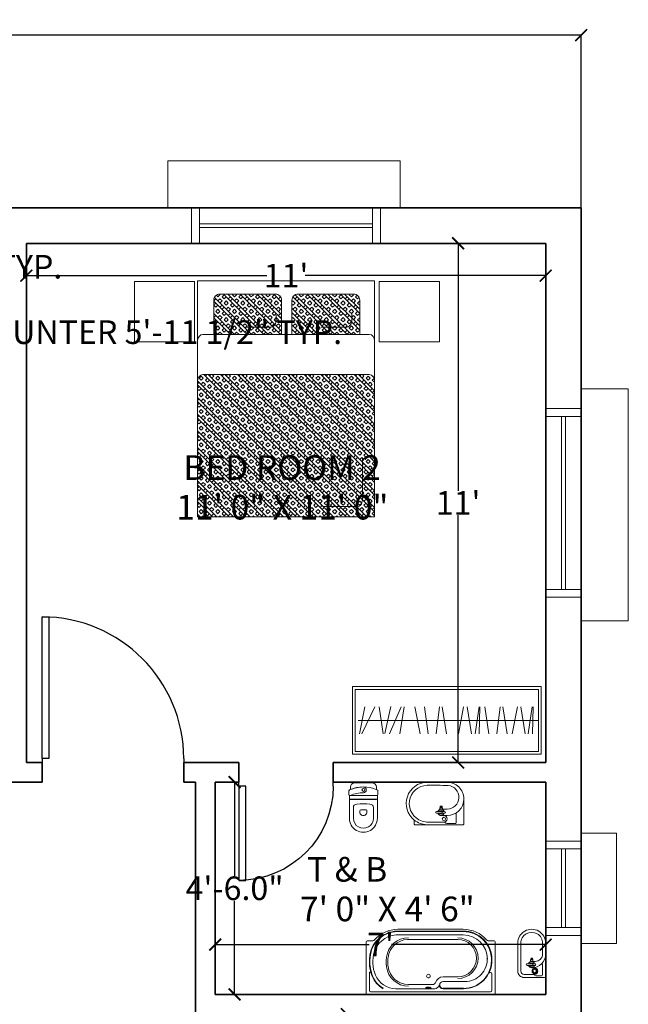
# Model space of a CAD drawing. Units: inches. Extents: x 844 to 2234, y 346 to 1084.
# Tile 93 of 93: x 2033 to 2188, y 828 to 1078. Entities that reach past the tile are written whole.
import ezdxf

# ---------------------------------------------------------------- set-up
doc = ezdxf.new("R2010")
doc.units = ezdxf.units.IN
doc.header["$MEASUREMENT"] = 0
for name, color, linetype, lineweight in [('A-ANNO-DIMS', 2, 'Continuous', 18), ('A-AREA-IDEN', 7, 'Continuous', 18), ('A-FLOR-FIXT', 8, 'Continuous', 18), ('A-WALL', 7, 'Continuous', 35), ('beds', 130, 'Continuous', 18), ('doors', 170, 'Continuous', 25), ('furniture', 8, 'Continuous', 18), ('windows', 1, 'Continuous', 18)]:
    doc.layers.add(name, color=color, linetype=linetype, lineweight=lineweight)
doc.styles.get("Standard").update_dxf_attribs({"font": 'arial.ttf'})
doc.dimstyles.get("Standard").update_dxf_attribs({"dimtxt": 6, "dimasz": 3, "dimexe": 0.18, "dimexo": 0.0625, "dimgap": 0.09, "dimtad": 0, "dimtih": 1, "dimtoh": 1, "dimdec": 1, "dimzin": 0, "dimdsep": 46, "dimlunit": 3, "dimtxsty": 'Standard', "dimblk": 'ARCHTICK', "dimcen": 0.09, "dimadec": 0, "dimazin": 0, "dimtfac": 1, "dimtdec": 1, "dimtofl": 0, "dimtmove": 0, "dimatfit": 3, "dimfxl": 1, "dimtolj": 1, "dimtzin": 0, "dimarcsym": 0})
pattern_1 = [(135, (-1377.70473, -125.71507), (-0.070710678, -0.070710678), []), (135, (-1377.68705, -125.69739), (-0.070710678, -0.070710678), []), (45, (-1377.70473, -125.71507), (-0.070710678, 0.070710678), [-0.025, 0.025]), (45, (-1377.72241, -125.69739), (-0.070710678, 0.070710678), [-0.025, 0.025]), (45, (-1377.74009, -125.67972), (-0.070710678, 0.070710678), [0.025, -0.025]), (45, (-1377.75776, -125.66204), (-0.070710678, 0.070710678), [0.025, -0.025]), (135, (-1377.66938, -125.67972), (-0.070710678, -0.070710678), [0.025, -0.025]), (135, (-1377.6517, -125.66204), (-0.070710678, -0.070710678), [0.025, -0.025])]

# ---------------------------------------------------------------- blocks, each defined once
blk = doc.blocks.new('*U2')
for p, q in [((0, 0), (0, -6)), ((36, 0), (36, -6))]:
    blk.add_line(p, q)
blk.add_lwpolyline([(0, 0), (0, 36), (1.75, 36), (1.75, 0)], close=True)
blk.add_arc((0, 0), 36, 0, 90)
blk = doc.blocks.new('*U4')
for p, q in [((0, 0), (0, -6)), ((24, 0), (24, -6))]:
    blk.add_line(p, q)
blk.add_lwpolyline([(0, 0), (0, 24), (1.75, 24), (1.75, 0)], close=True)
blk.add_arc((0, 0), 24, 0, 90)
blk = doc.blocks.new('MAT-P10')
h = blk.add_hatch()
h.set_pattern_fill('BOX', color=256, scale=0.1, angle=45, style=0)
h.set_pattern_definition(pattern_1)
h.paths.add_polyline_path([(-0.1565, 1.4605), (0.417, 1.4605), (0.417, 1.7513, 0.414214), (0.367, 1.8013), (-0.1065, 1.8013, 0.414214), (-0.1565, 1.7513)])
h.paths.add_polyline_path([(0.5052, 1.4604), (1.0792, 1.4604), (1.0792, 1.7513, 0.414214), (1.0292, 1.8013), (0.5552, 1.8013, 0.414214), (0.5052, 1.7513)])
h = blk.add_hatch()
h.set_pattern_fill('BOX', color=256, scale=0.1, angle=45, style=0)
h.set_pattern_definition(pattern_1)
edge = h.paths.add_edge_path()
edge.add_line((1.2049, -0.085), (1.2049, 1.0625))
edge.add_ellipse((1.1608, 1.0627), major_axis=(0, 0.0568), ratio=0.776379, start_angle=270, end_angle=360)
edge.add_line((1.1608, 1.1195), (-0.251, 1.1195))
edge.add_ellipse((-0.251, 1.0627), major_axis=(0, 0.0568), ratio=0.776379, start_angle=0, end_angle=88.13958)
edge.add_line((-0.2951, 1.0641), (-0.2951, -0.085))
edge.add_line((-0.2951, -0.085), (1.2049, -0.085))
for p, q in [((-0.251, 1.4605), (1.1608, 1.4604)), ((-0.251, 1.1195), (1.1608, 1.1195)), ((1.1017, 0.406), (1.1017, 0.0572)), ((1.0576, 0.0004), (0.7754, 0.0004))]:
    blk.add_line(p, q)
for points in [[(-0.8301, 1.9091), (-0.3191, 1.9091), (-0.3191, 1.3981), (-0.8301, 1.3981)], [(1.2049, -0.085), (-0.2951, -0.085), (-0.2951, 1.9151), (1.2049, 1.915)], [(1.2441, 1.9091), (1.755, 1.9091), (1.755, 1.3981), (1.2441, 1.3981)]]:
    blk.add_lwpolyline(points, close=True)
for points in [[(0.417, 1.4604), (0.417, 1.7513, 0.414214), (0.367, 1.8013), (-0.1065, 1.8013, 0.414214), (-0.1565, 1.7513), (-0.1565, 1.4604)], [(1.0792, 1.4603), (1.0792, 1.7513, 0.414214), (1.0292, 1.8013), (0.5552, 1.8013, 0.414214), (0.5052, 1.7513), (0.5052, 1.4604)], [(0.3702, 1.6242), (0.3702, 1.5715, -0.414214), (0.3202, 1.5215), (0.1113, 1.5215)], [(1.0117, 1.6438), (1.0117, 1.5715, -0.414214), (0.9617, 1.5215), (0.7528, 1.5215)]]:
    blk.add_lwpolyline(points, format="xyb")
at = {"extrusion": (0, 0, -1)}
for centre, start_param, end_param in [((-0.251, 1.4036), 4.712389, 6.283185), ((1.1608, 1.4036), 0, 1.570796), ((-0.251, 1.0627), 4.712389, 6.283185), ((1.1608, 1.0627), 0, 1.570796), ((1.0576, 0.0572), 1.570796, 3.141593), ((1.0576, 0.0572), 1.570796, 3.141593)]:
    blk.add_ellipse(centre, major_axis=(0, 0.0568), ratio=0.776379, start_param=start_param, end_param=end_param, dxfattribs=at)
blk = doc.blocks.new('A$C7A17768A')
for p, q in [((-2.8, 0), (0, 0)), ((-2.8, -1), (-2.8, 0)), ((0, -1), (0, 0)), ((-2.76, -0.04), (-0.04, -0.04)), ((-2.76, -0.96), (-2.76, -0.04)), ((-0.04, -0.96), (-0.04, -0.04)), ((-2.617, -0.3), (-2.694, -0.7)), ((-2.66, -0.7), (-2.466, -0.3)), ((-2.403, -0.3), (-2.342, -0.7)), ((-2.229, -0.296), (-2.317, -0.696)), ((-2.074, -0.3), (-2.25, -0.7)), ((-2.096, -0.7), (-2.033, -0.3)), ((-1.875, -0.3), (-1.796, -0.7)), ((-1.732, -0.3), (-1.675, -0.7)), ((-1.555, -0.7), (-1.507, -0.3)), ((-1.467, -0.3), (-1.403, -0.7)), ((-1.227, -0.7), (-1.151, -0.3)), ((-1.098, -0.3), (-1.034, -0.7)), ((-0.98, -0.7), (-0.921, -0.3)), ((-0.908, -0.3), (-0.919, -0.7)), ((-0.834, -0.3), (-0.777, -0.7)), ((-0.657, -0.7), (-0.61, -0.3)), ((-0.57, -0.3), (-0.505, -0.7)), ((-0.429, -0.7), (-0.353, -0.3)), ((-0.301, -0.3), (-0.237, -0.7)), ((-0.192, -0.7), (-0.133, -0.3)), ((-0.12, -0.3), (-0.131, -0.7)), ((-0.04, -0.5), (-2.716, -0.5)), ((-2.8, -1), (0, -1)), ((-2.76, -0.96), (-0.04, -0.96))]:
    blk.add_line(p, q)
blk = doc.blocks.new('2SABICO')
at = {"color": 0, "linetype": 'ByBlock'}
for p, q in [((0.478, 0.195), (0.089, 0.195)), ((0.478, 0.152), (0.089, 0.152)), ((0, 0.106), (0, 0)), ((0, 0), (0, -0.18)), ((0.043, -0.039), (0.043, 0.106)), ((0.135, 0), (0.135, -0.003)), ((0.168, 0.064), (0.168, -0.015)), ((0.192, 0.064), (0.192, -0.015)), ((0.221, 0.012), (0.222, 0.012)), ((0.223, 0.016), (0.223, -0.016)), ((0.224, 0.017), (0.245, 0.017)), ((0.246, 0.016), (0.246, -0.016)), ((0.25, 0.014), (0.246, 0.014)), ((0.26, 0.01), (0.268, 0.01)), ((0.268, -0.01), (0.268, 0.01)), ((0.268, 0.01), (0.269, 0.009)), ((0.269, -0.009), (0.269, 0.009)), ((0.023, -0.057), (0.023, -0.135)), ((0.135, 0), (0.135, -0.039)), ((0.168, -0.015), (0.192, -0.015)), ((0.168, -0.015), (0.168, -0.046)), ((0.192, -0.015), (0.192, -0.046)), ((0.221, -0.012), (0.222, -0.012)), ((0.224, -0.017), (0.245, -0.017)), ((0.225, -0.017), (0.225, -0.047)), ((0.25, -0.014), (0.246, -0.014)), ((0.26, -0.01), (0.268, -0.01)), ((0.268, -0.01), (0.269, -0.009)), ((0.015, -0.195), (0.478, -0.195)), ((0.038, -0.15), (0.179, -0.15)), ((0.33, -0.152), (0.478, -0.152))]:
    blk.add_line(p, q, dxfattribs=at)
for radius in [0.035, 0.023]:
    blk.add_circle((0.089, -0.039), radius, dxfattribs=at)
for centre, radius, start, end in [((0.089, 0.106), 0.089, 90, 180), ((0.089, 0.106), 0.046, 90, 180), ((0.478, 0), 0.195, 270, 90), ((0.478, 0), 0.152, 270, 90), ((0.18, 0), 0.045, 105.6643, 180), ((0.18, 0), 0.042, 106.8152, 252.6853), ((0.18, 0), 0.0235, 121.1327, 237.8651), ((0.18, 0.064), 0.0121, 0, 180), ((0.18, 0), 0.045, 17.0576, 74.3357), ((0.18, 0), 0.042, 287.3147, 73.1848), ((0.18, 0), 0.0235, 302.1349, 58.8673), ((0.221, 0.013), 0.001, 197.9471, 270), ((0.222, 0.013), 0.001, 270, 0), ((0.224, 0.016), 0.001, 90, 180), ((0.245, 0.016), 0.001, 0, 90), ((0.25, 0), 0.0143, 270, 90), ((0.041, -0.057), 0.018, 99.5941, 180), ((0.038, -0.135), 0.015, 180, 270), ((0.037, -0.033), 0.006, 279.5941, 0), ((0.089, -0.039), 0.046, 180, 360), ((0.326, -0.003), 0.191, 180, 270), ((0.18, -0.046), 0.0125, 180, 0), ((0.179, -0.14), 0.01, 270, 42.9682), ((0.221, -0.013), 0.001, 90, 162.0529), ((0.222, -0.013), 0.001, 0, 90), ((0.224, -0.016), 0.001, 180, 270), ((0.33, -0.047), 0.105, 180, 270), ((0.245, -0.016), 0.001, 270, 0), ((0.015, -0.18), 0.015, 180, 270)]:
    blk.add_arc(centre, radius, start, end, dxfattribs=at)
blk = doc.blocks.new('2SAINCO')
at = {"color": 0, "linetype": 'ByBlock'}
for p, q in [((0.06, 0.181), (0.085, 0.181)), ((0.114, 0.203), (0.165, 0.203)), ((0.496, 0.195), (0.178, 0.195)), ((0.18, -0.188), (0.18, 0.188)), ((0.231, 0.185), (0.231, -0.185)), ((0.234, 0.185), (0.234, -0.185)), ((0.496, 0.14), (0.347, 0.14)), ((0, -0.121), (0, 0.121)), ((0.394, 0.05), (0.407, 0.05)), ((0.394, -0.05), (0.407, -0.05)), ((0.06, -0.181), (0.085, -0.181)), ((0.114, -0.201), (0.165, -0.201)), ((0.114, -0.203), (0.165, -0.203)), ((0.496, -0.195), (0.178, -0.195)), ((0.496, -0.14), (0.347, -0.14))]:
    blk.add_line(p, q, dxfattribs=at)
blk.add_circle((0.1, 0), 0.02, dxfattribs=at)
for centre, radius, start, end in [((0.06, 0.121), 0.06, 90, 180), ((0.517, 0), 0.46, 155.909, 204.091), ((0.085, 0.196), 0.015, 270, 344.534), ((0.114, 0.188), 0.015, 90, 164.534), ((0.165, 0.188), 0.015, 0, 90), ((0.221, 0.185), 0.01, 0, 90), ((0.224, 0.185), 0.01, 0, 90), ((0.347, 0.09), 0.05, 90, 177.3546), ((0.496, 0), 0.195, 270, 90), ((0.496, 0), 0.14, 270, 90), ((0.1, 0), 0.0405, 360, 180), ((0.517, 0), 0.458, 180, 204.67), ((0.66, 0.008), 0.52, 180.891, 201.3823), ((2.295, 0), 2, 177.3546, 182.6454), ((0.677, 0), 0.3, 172.9459, 187.0541), ((0.394, 0.035), 0.015, 90, 172.9459), ((0.407, 0), 0.05, 270, 90), ((0.06, -0.121), 0.06, 180, 270), ((0.347, -0.09), 0.05, 182.6454, 270), ((0.394, -0.035), 0.015, 187.0541, 270), ((0.085, -0.196), 0.015, 15.466, 90), ((0.114, -0.188), 0.015, 195.466, 270), ((0.114, -0.188), 0.013, 195.466, 270), ((0.165, -0.188), 0.013, 270, 30), ((0.165, -0.188), 0.015, 270, 0), ((0.221, -0.185), 0.01, 270, 0), ((0.224, -0.185), 0.01, 270, 0)]:
    blk.add_arc(centre, radius, start, end, dxfattribs=at)
blk = doc.blocks.new('2SABACO')
at = {"color": 0}
for p, q in [((1.341, 0.831), (0.407, 0.831)), ((1.341, 0.91), (0.429, 0.91)), ((1.341, 0.885), (0.429, 0.885)), ((1.341, 0.879), (0.429, 0.879)), ((-0.015, 0.735), (-0.015, 0.015)), ((0, 0.75), (0.08, 0.75)), ((1.263, 0.769), (0.562, 0.769)), ((1.77, 0.75), (1.69, 0.75)), ((1.785, 0.015), (1.785, 0.735)), ((0.03, 0.302), (0.03, 0.053)), ((1.74, 0.053), (1.74, 0.286)), ((0.578, 0.139), (0.911, 0.139)), ((1.263, 0.245), (1.06, 0.245)), ((1.363, 0.181), (1.06, 0.181)), ((0, 0), (1.77, 0)), ((0.048, 0.035), (1.722, 0.035)), ((0.401, 0.08), (0.942, 0.08)), ((1.343, 0.086), (1.06, 0.086)), ((1.343, 0.079), (1.06, 0.079))]:
    blk.add_line(p, q, dxfattribs=at)
blk.add_circle((0.855, 0.256), 0.026, dxfattribs=at)
for centre, radius, start, end in [((0.428, 0.49), 0.395, 98.9726, 181.1954), ((0.428, 0.49), 0.389, 98.9726, 181.2301), ((0.425, 0.49), 0.342, 93.1008, 168.0202), ((0.429, 0.48), 0.43, 90, 139.2943), ((0.429, 0.48), 0.405, 90, 98.9726), ((0.429, 0.48), 0.399, 90, 98.9726), ((1.341, 0.48), 0.43, 40.7057, 90), ((1.341, 0.485), 0.401, 359.4627, 90), ((1.341, 0.485), 0.394, 3.5237, 90), ((1.341, 0.495), 0.336, 0, 90), ((0, 0.735), 0.015, 90, 180), ((0.08, 0.78), 0.03, 270, 319.2943), ((0.578, 0.481), 0.311, 90, 172.609), ((0.578, 0.481), 0.288, 93.3767, 172.609), ((1.263, 0.507), 0.285, 270, 90), ((1.263, 0.507), 0.262, 270, 90), ((1.69, 0.78), 0.03, 220.7057, 270), ((1.77, 0.735), 0.015, 0, 90), ((0.559, 0.454), 0.48, 163.1286, 202.3619), ((0.559, 0.454), 0.528, 177.0415, 202.3619), ((0.559, 0.454), 0.521, 177.0156, 202.3619), ((0.79, 0.454), 0.525, 172.609, 180), ((0.79, 0.454), 0.525, 180, 187.391), ((0.79, 0.454), 0.502, 172.609, 180), ((0.79, 0.454), 0.502, 180, 187.391), ((1.343, 0.477), 0.392, 270, 4.5675), ((1.343, 0.477), 0.398, 270, 0.539), ((1.363, 0.495), 0.314, 270, 2.2815), ((0.042, 0.302), 0.0116, 16.3184, 180.0001), ((0.578, 0.427), 0.311, 187.391, 270), ((0.578, 0.427), 0.288, 187.391, 270), ((1.718, 0.286), 0.0222, 0, 152.9966), ((0.401, 0.389), 0.357, 202.3619, 239.8287), ((0.401, 0.389), 0.351, 202.3619, 239.2093), ((0.401, 0.389), 0.309, 202.3619, 270), ((0.911, 0.183), 0.045, 270, 341.2369), ((1.06, 0.133), 0.112, 90, 161.2369), ((1.06, 0.133), 0.0475, 90, 270), ((0, 0.015), 0.015, 180, 270), ((0.048, 0.053), 0.018, 180, 270), ((0.559, 0.454), 0.48, 250.7818, 251.0555), ((0.821, 0.092), 0.00282, 119.7759, 180), ((0.821, 0.092), 0.00282, 180, 240.2241), ((0.837, 0.064), 0.0347, 103.3326, 119.7759), ((0.835, 0.025), 0.071, 96.5949, 102.1924), ((0.837, 0.12), 0.0347, 240.2241, 256.6674), ((0.847, -0.08), 0.177, 92.7417, 96.5949), ((0.848, 0.02), 0.0808, 95.6065, 103.3326), ((0.848, 0.164), 0.0808, 256.6674, 264.3935), ((0.855, -0.252), 0.349, 90, 92.7417), ((0.855, -0.053), 0.153, 90, 95.6065), ((0.855, 0.237), 0.153, 264.3935, 270), ((0.855, -0.053), 0.153, 84.3935, 90), ((0.855, -0.252), 0.349, 87.2583, 90), ((0.855, 0.237), 0.153, 270, 275.6065), ((0.862, 0.02), 0.0808, 76.6674, 84.3935), ((0.862, 0.164), 0.0808, 275.6065, 283.3326), ((0.863, -0.08), 0.177, 83.4051, 87.2583), ((0.873, 0.064), 0.0347, 60.2241, 76.6674), ((0.873, 0.12), 0.0347, 283.3326, 299.7759), ((0.875, 0.025), 0.071, 77.8076, 83.4051), ((0.889, 0.092), 0.00282, 360, 60.2241), ((0.889, 0.092), 0.00282, 299.7759, 360), ((0.942, 0.145), 0.065, 270, 349.4977), ((1.06, 0.133), 0.054, 180, 270), ((1.722, 0.053), 0.018, 270, 0), ((1.77, 0.015), 0.015, 270, 0)]:
    blk.add_arc(centre, radius, start, end, dxfattribs=at)
blk = doc.blocks.new('2SALACO2')
at = {"color": 0}
for p, q in [((0, 0), (-0.392, 0)), ((0.28, 0), (0, 0)), ((-0.402, -0.01), (-0.402, -0.36)), ((-0.293, -0.026), (-0.293, -0.15)), ((-0.283, -0.016), (-0.166, -0.016)), ((-0.169, -0.128), (-0.085, -0.128)), ((-0.112, -0.035), (-0.133, -0.035)), ((-0.124, -0.035), (0.09, -0.035)), ((0.29, -0.01), (0.29, -0.064)), ((-0.102, -0.219), (-0.169, -0.219)), ((-0.1, -0.161), (-0.131, -0.161)), ((-0.1, -0.186), (-0.131, -0.186)), ((-0.102, -0.217), (-0.102, -0.234)), ((-0.07, -0.216), (-0.101, -0.216)), ((-0.07, -0.235), (-0.101, -0.235)), ((-0.1, -0.161), (-0.1, -0.186)), ((-0.021, -0.161), (-0.1, -0.161)), ((-0.021, -0.186), (-0.1, -0.186)), ((-0.098, -0.214), (-0.098, -0.216)), ((-0.097, -0.239), (-0.098, -0.241)), ((-0.098, -0.241), (-0.098, -0.248)), ((-0.098, -0.241), (-0.073, -0.241)), ((-0.073, -0.248), (-0.098, -0.248)), ((-0.097, -0.235), (-0.097, -0.239)), ((-0.074, -0.239), (-0.097, -0.239)), ((-0.097, -0.248), (-0.097, -0.256)), ((-0.073, -0.256), (-0.097, -0.256)), ((-0.097, -0.256), (-0.094, -0.257)), ((-0.077, -0.257), (-0.094, -0.257)), ((-0.073, -0.256), (-0.077, -0.257)), ((-0.074, -0.235), (-0.074, -0.239)), ((-0.074, -0.239), (-0.073, -0.241)), ((-0.073, -0.214), (-0.073, -0.216)), ((-0.073, -0.241), (-0.073, -0.248)), ((-0.073, -0.248), (-0.073, -0.256)), ((-0.069, -0.217), (-0.069, -0.234))]:
    blk.add_line(p, q, dxfattribs=at)
blk.add_lwpolyline([(-0.402, -0.36, 0.423787), (-0.161, -0.593, 0.423787)], format="xyb", dxfattribs=at)
blk.add_circle((-0.124, -0.081), 0.023, dxfattribs=at)
for centre, radius, start, end in [((-0.392, -0.01), 0.01, 90, 180), ((0.28, -0.01), 0.01, 0, 90), ((-0.169, -0.36), 0.233, 90, 180), ((-0.283, -0.026), 0.01, 90, 180), ((-0.124, -0.081), 0.0462, 90, 270), ((-0.166, -0.046), 0.03, 31.2573, 90), ((-0.133, -0.026), 0.009, 211.2573, 270), ((-0.085, -0.173), 0.042, 16.8152, 162.6853), ((-0.085, -0.173), 0.0458, 15.3964, 90), ((0.09, -0.29), 0.255, 68.9449, 90), ((0.105, -0.295), 0.255, 271.0077, 72.4499), ((0.105, -0.297), 0.297, 271.4871, 51.4524), ((0.105, -0.297), 0.297, 51.4524, 87.1707), ((-0.169, -0.383), 0.164, 90, 265.4963), ((-0.285, -0.15), 0.008, 180, 299.1062), ((-0.131, -0.173), 0.0125, 90, 270), ((-0.085, -0.173), 0.042, 197.3147, 343.1848), ((-0.085, -0.173), 0.0235, 31.1327, 147.8651), ((-0.085, -0.173), 0.0235, 212.1349, 328.8673), ((-0.101, -0.217), 0.001, 90, 180), ((-0.101, -0.234), 0.001, 180, 270), ((-0.085, -0.173), 0.0458, 289.9182, 344.6036), ((-0.07, -0.217), 0.001, 0, 90), ((-0.07, -0.234), 0.001, 270, 0), ((-0.021, -0.173), 0.0121, 270, 90), ((0.021, 4.449), 5, 267.6742, 271.0081), ((-0.017, 4.405), 5, 268.3511, 271.4874)]:
    blk.add_arc(centre, radius, start, end, dxfattribs=at)
blk = doc.blocks.new('_ArchTick')
at = {"color": 0, "linetype": 'ByBlock', "const_width": 0.15}
blk.add_lwpolyline([(-0.5, -0.5), (0.5, 0.5)], dxfattribs=at)
blk = doc.blocks.new('*D60')
at = {"layer": 'A-ANNO-DIMS', "color": 0, "lineweight": -2, "transparency": 16777216}
for p, q in [((2144.84, 1021.46), (2144.84, 958.56)), ((2144.91, 1021.46), (2145.02, 1021.46)), ((2144.84, 889.46), (2144.84, 952.35)), ((2144.91, 889.46), (2145.02, 889.46))]:
    blk.add_line(p, q, dxfattribs=at)
at = {"layer": 'Defpoints', "color": 0, "transparency": 16777216}
for p in [(2144.84, 1021.46), (2144.84, 889.46), (2144.84, 889.46)]:
    blk.add_point(p, dxfattribs=at)
at = {"layer": 'A-ANNO-DIMS', "color": 0, "lineweight": -2, "transparency": 16777216, "xscale": 3, "yscale": 3, "zscale": 3}
for p, rotation in [((2144.84, 1021.46), 90), ((2144.84, 889.46), 270)]:
    blk.add_blockref('_ArchTick', p, dxfattribs=dict(at, rotation=rotation))
at = {"layer": 'A-ANNO-DIMS', "color": 0, "transparency": 16777216, "insert": (2144.84, 955.46), "char_height": 6, "attachment_point": 5}
blk.add_mtext("\\A1;11'", dxfattribs=at)
blk = doc.blocks.new('*D66')
at = {"layer": 'A-ANNO-DIMS', "color": 0, "lineweight": -2, "transparency": 16777216}
for p, q in [((2035.1, 1019.03), (2035.1, 1013.06)), ((2167.1, 1019.03), (2167.1, 1013.06)), ((2035.1, 1013.24), (2096.2, 1013.24)), ((2167.1, 1013.24), (2106, 1013.24))]:
    blk.add_line(p, q, dxfattribs=at)
at = {"layer": 'Defpoints', "color": 0, "transparency": 16777216}
for p in [(2035.1, 1019.1), (2167.1, 1019.1), (2167.1, 1013.24)]:
    blk.add_point(p, dxfattribs=at)
at = {"layer": 'A-ANNO-DIMS', "color": 0, "lineweight": -2, "transparency": 16777216, "xscale": 3, "yscale": 3, "zscale": 3, "rotation": 180}
blk.add_blockref('_ArchTick', (2035.1, 1013.24), dxfattribs=at)
at = {"layer": 'A-ANNO-DIMS', "color": 0, "lineweight": -2, "transparency": 16777216, "xscale": 3, "yscale": 3, "zscale": 3}
blk.add_blockref('_ArchTick', (2167.1, 1013.24), dxfattribs=at)
at = {"layer": 'A-ANNO-DIMS', "color": 0, "transparency": 16777216, "insert": (2101.1, 1013.24), "char_height": 6, "attachment_point": 5}
blk.add_mtext("\\A1;11'", dxfattribs=at)
blk = doc.blocks.new('*D74')
at = {"layer": 'A-ANNO-DIMS', "color": 0, "lineweight": -2, "transparency": 16777216}
for p, q in [((2086.16, 884.46), (2088.2, 884.46)), ((2088.02, 884.46), (2088.02, 860.61)), ((2088.02, 830.46), (2088.02, 854.3)), ((2086.16, 830.46), (2088.2, 830.46))]:
    blk.add_line(p, q, dxfattribs=at)
at = {"layer": 'Defpoints', "color": 0, "transparency": 16777216}
for p in [(2086.1, 884.46), (2086.1, 830.46), (2088.02, 830.46)]:
    blk.add_point(p, dxfattribs=at)
at = {"layer": 'A-ANNO-DIMS', "color": 0, "lineweight": -2, "transparency": 16777216, "xscale": 3, "yscale": 3, "zscale": 3}
for p, rotation in [((2088.02, 884.46), 90), ((2088.02, 830.46), 270)]:
    blk.add_blockref('_ArchTick', p, dxfattribs=dict(at, rotation=rotation))
at = {"layer": 'A-ANNO-DIMS', "color": 0, "transparency": 16777216, "insert": (2088.02, 857.46), "char_height": 6, "attachment_point": 5}
blk.add_mtext('\\A1;4\'-6.0"', dxfattribs=at)
blk = doc.blocks.new('*D75')
at = {"layer": 'A-ANNO-DIMS', "color": 0, "lineweight": -2, "transparency": 16777216}
for p, q in [((2083.1, 847.39), (2083.1, 842.96)), ((2167.1, 847.39), (2167.1, 842.96)), ((2083.1, 843.14), (2122.27, 843.14)), ((2167.1, 843.14), (2127.93, 843.14))]:
    blk.add_line(p, q, dxfattribs=at)
at = {"layer": 'Defpoints', "color": 0, "transparency": 16777216}
for p in [(2083.1, 847.46), (2167.1, 847.46), (2083.1, 843.14)]:
    blk.add_point(p, dxfattribs=at)
at = {"layer": 'A-ANNO-DIMS', "color": 0, "lineweight": -2, "transparency": 16777216, "xscale": 3, "yscale": 3, "zscale": 3, "rotation": 180}
blk.add_blockref('_ArchTick', (2083.1, 843.14), dxfattribs=at)
at = {"layer": 'A-ANNO-DIMS', "color": 0, "lineweight": -2, "transparency": 16777216, "xscale": 3, "yscale": 3, "zscale": 3}
blk.add_blockref('_ArchTick', (2167.1, 843.14), dxfattribs=at)
at = {"layer": 'A-ANNO-DIMS', "color": 0, "transparency": 16777216, "insert": (2125.1, 843.14), "char_height": 6, "attachment_point": 5}
blk.add_mtext("\\A1;7'", dxfattribs=at)
blk = doc.blocks.new('*D86')
at = {"layer": 'A-ANNO-DIMS', "color": 0, "lineweight": -2, "transparency": 16777216}
for p, q in [((1697.1, 1030.52), (1697.1, 1074.57)), ((1697.1, 1074.39), (1920.38, 1074.39)), ((2176.1, 1074.39), (1952.82, 1074.39)), ((2176.1, 1030.52), (2176.1, 1074.57))]:
    blk.add_line(p, q, dxfattribs=at)
at = {"layer": 'Defpoints', "color": 0, "transparency": 16777216}
for p in [(2176.1, 1074.39), (1697.1, 1030.46), (2176.1, 1030.46)]:
    blk.add_point(p, dxfattribs=at)
at = {"layer": 'A-ANNO-DIMS', "color": 0, "lineweight": -2, "transparency": 16777216, "xscale": 3, "yscale": 3, "zscale": 3, "rotation": 180}
blk.add_blockref('_ArchTick', (1697.1, 1074.39), dxfattribs=at)
at = {"layer": 'A-ANNO-DIMS', "color": 0, "lineweight": -2, "transparency": 16777216, "xscale": 3, "yscale": 3, "zscale": 3}
blk.add_blockref('_ArchTick', (2176.1, 1074.39), dxfattribs=at)
at = {"layer": 'A-ANNO-DIMS', "color": 0, "transparency": 16777216, "insert": (1936.6, 1074.39), "char_height": 6, "attachment_point": 5}
blk.add_mtext('\\A1;39\'-11.0"', dxfattribs=at)
blk = doc.blocks.new('WIN-48IN')
for p, q in [((0, 9), (0, 21)), ((0, 21), (59, 21)), ((59, 9), (59, 21)), ((6, 9), (0, 9)), ((54, 9), (6, 9)), ((6, 9), (6, 0)), ((8, 9), (8, 0)), ((52, 0), (52, 9)), ((54, 0), (54, 9)), ((54, 9), (59, 9)), ((8, 5), (52, 5)), ((8, 4), (52, 4)), ((6, 0), (54, 0))]:
    blk.add_line(p, q)
blk = doc.blocks.new('WIN-24IN')
for p, q in [((9, 28), (0, 28)), ((0, 0), (0, 28)), ((9, 26), (9, 28)), ((18, 26), (9, 26)), ((9, 26), (9, 2)), ((18, 2), (18, 26)), ((18, 24), (9, 24)), ((13, 4), (13, 24)), ((14, 4), (14, 24)), ((9, 4), (18, 4)), ((9, 2), (18, 2)), ((9, 2), (9, 0)), ((9, 0), (0, 0))]:
    blk.add_line(p, q)
blk = doc.blocks.new('*D116')
at = {"layer": 'A-ANNO-DIMS', "color": 0, "lineweight": -2, "transparency": 16777216}
for p, q in [((2121.39, 825.46), (2116.36, 825.46)), ((2116.54, 825.46), (2116.54, 820.36)), ((2116.54, 808.88), (2116.54, 813.98)), ((2121.39, 808.88), (2116.36, 808.88))]:
    blk.add_line(p, q, dxfattribs=at)
at = {"layer": 'Defpoints', "color": 0, "transparency": 16777216}
for p in [(2121.46, 825.46), (2116.54, 808.88), (2121.46, 808.88)]:
    blk.add_point(p, dxfattribs=at)
at = {"layer": 'A-ANNO-DIMS', "color": 0, "lineweight": -2, "transparency": 16777216, "xscale": 3, "yscale": 3, "zscale": 3}
for p, rotation in [((2116.54, 825.46), 90), ((2116.54, 808.88), 270)]:
    blk.add_blockref('_ArchTick', p, dxfattribs=dict(at, rotation=rotation))
at = {"layer": 'A-ANNO-DIMS', "color": 0, "transparency": 16777216, "insert": (2116.54, 817.17), "char_height": 6, "attachment_point": 5}
blk.add_mtext('\\A1;1\'-4 1/2" TYP.', dxfattribs=at)
blk = doc.blocks.new('*D129')
at = {"layer": 'A-ANNO-DIMS', "color": 0, "lineweight": -2, "transparency": 16777216}
for p, q in [((1943.95, 1009.51), (1943.95, 998.7)), ((2015.23, 1009.51), (2015.23, 998.7)), ((1943.95, 998.88), (2015.23, 998.88)), ((2015.23, 998.88), (2018.23, 998.88))]:
    blk.add_line(p, q, dxfattribs=at)
at = {"layer": 'Defpoints', "color": 0, "transparency": 16777216}
for p in [(1943.95, 1009.57), (2015.23, 1009.57), (2015.23, 998.88)]:
    blk.add_point(p, dxfattribs=at)
at = {"layer": 'A-ANNO-DIMS', "color": 0, "lineweight": -2, "transparency": 16777216, "xscale": 3, "yscale": 3, "zscale": 3, "rotation": 180}
blk.add_blockref('_ArchTick', (1943.95, 998.88), dxfattribs=at)
at = {"layer": 'A-ANNO-DIMS', "color": 0, "lineweight": -2, "transparency": 16777216, "xscale": 3, "yscale": 3, "zscale": 3}
blk.add_blockref('_ArchTick', (2015.23, 998.88), dxfattribs=at)
at = {"layer": 'A-ANNO-DIMS', "color": 0, "transparency": 16777216, "insert": (2067.78, 998.88), "char_height": 6, "attachment_point": 5}
blk.add_mtext('\\A1;COUNTER 5\'-11 1/2" TYP.', dxfattribs=at)
blk = doc.blocks.new('*D130')
at = {"layer": 'A-ANNO-DIMS', "color": 0, "lineweight": -2, "transparency": 16777216}
for p, q in [((2015.29, 1021.46), (2026.1, 1021.46)), ((2025.92, 1021.46), (2025.92, 1018.67)), ((2025.92, 1009.57), (2025.92, 1012.36)), ((2015.29, 1009.57), (2026.1, 1009.57))]:
    blk.add_line(p, q, dxfattribs=at)
at = {"layer": 'Defpoints', "color": 0, "transparency": 16777216}
for p in [(2015.23, 1021.46), (2025.92, 1021.46), (2015.23, 1009.57)]:
    blk.add_point(p, dxfattribs=at)
at = {"layer": 'A-ANNO-DIMS', "color": 0, "lineweight": -2, "transparency": 16777216, "xscale": 3, "yscale": 3, "zscale": 3}
for p, rotation in [((2025.92, 1021.46), 90), ((2025.92, 1009.57), 270)]:
    blk.add_blockref('_ArchTick', p, dxfattribs=dict(at, rotation=rotation))
at = {"layer": 'A-ANNO-DIMS', "color": 0, "transparency": 16777216, "insert": (2025.92, 1015.51), "char_height": 6, "attachment_point": 5}
blk.add_mtext('\\A1;1\'-0" TYP.', dxfattribs=at)

msp = doc.modelspace()

# ---------------------------------------------------------------- linework, layer by layer
at = {"layer": 'A-WALL'}
for p, q in [((1697.1, 1030.46), (2176.1, 1030.46)), ((2176.1, 1030.46), (2176.1, 435.46)), ((2035.1, 1021.46), (2035.1, 889.46)), ((2035.1, 1021.46), (2167.1, 1021.46)), ((2167.1, 1021.46), (2167.1, 889.46)), ((2035.1, 889.46), (2039.1, 889.46)), ((2039.1, 889.46), (2039.1, 884.46)), ((2075.1, 889.46), (2089.1, 889.46)), ((2075.1, 889.46), (2075.1, 884.46)), ((2089.1, 884.46), (2089.1, 889.46)), ((2113.1, 889.46), (2167.1, 889.46)), ((2113.1, 884.46), (2113.1, 889.46)), ((1987.1, 884.46), (2039.1, 884.46)), ((2075.1, 884.46), (2078.1, 884.46)), ((2078.1, 884.46), (2078.1, 795.46)), ((2083.1, 884.46), (2089.1, 884.46)), ((2083.1, 884.46), (2083.1, 830.46)), ((2113.1, 884.46), (2167.1, 884.46)), ((2167.1, 884.46), (2167.1, 830.46)), ((2167.1, 830.46), (2083.1, 830.46))]:
    msp.add_line(p, q, dxfattribs=at)

# ---------------------------------------------------------------- block references
at = {"layer": 'A-FLOR-FIXT', "xscale": 18.21101258924898, "yscale": 18.21101258924898, "zscale": 18.21101258924898}
for name, p, rotation in [('2SAINCO', (2120.76, 884.29), 270), ('2SALACO2', (2138.98, 873.62), 180), ('2SABICO', (2163.55, 834.78), 89.99999999999999)]:
    msp.add_blockref(name, p, dxfattribs=dict(at, rotation=rotation))
msp.add_blockref('2SABACO', (2121.73, 830.46), dxfattribs=at)
at = {"layer": 'beds', "xscale": 29.99962925113936, "yscale": 29.99962925113936, "zscale": 29.99962925113936}
msp.add_blockref('MAT-P10', (2087.45, 954.49), dxfattribs=at)
at = {"layer": 'doors'}
msp.add_blockref('*U2', (2039.1, 890.46), dxfattribs=at)
at = {"layer": 'doors', "xscale": -1, "rotation": 180}
msp.add_blockref('*U4', (2089.1, 883.46), dxfattribs=at)
at = {"layer": 'furniture', "xscale": 17.14285714285603, "yscale": 17.14285714285603, "zscale": 17.14285714285603}
msp.add_blockref('A$C7A17768A', (2165.96, 908.73), dxfattribs=at)
at = {"layer": 'windows'}
msp.add_blockref('WIN-48IN', (2071.1, 1021.46), dxfattribs=at)
at = {"layer": 'windows', "extrusion": (0, 0, -1), "zscale": -1, "rotation": 90.00000000000318}
msp.add_blockref('WIN-48IN', (-2167.1, 925.46), dxfattribs=at)
at = {"layer": 'windows', "rotation": 180}
msp.add_blockref('WIN-24IN', (2185.1, 871.45), dxfattribs=at)

# ---------------------------------------------------------------- texts
at = {"layer": 'A-AREA-IDEN'}
for s, height, p in [('BED ROOM 2', 6.269, (2075, 961.3)), (' 11\' 0" X 11\' 0"', 6.2688, (2071.3, 951.23)), ('T & B', 6.269, (2106.43, 859.14)), (' 7\' 0" X 4\' 6"', 6.2688, (2102.73, 849.07))]:
    msp.add_text(s, height=height, dxfattribs=at).set_placement(p)

# ---------------------------------------------------------------- dimensions: what is measured, and where the dimension line sits
at = {"layer": 'A-ANNO-DIMS'}
for base, p1, p2, picture, middle in [((2176.1, 1074.39), (1697.1, 1030.46), (2176.1, 1030.46), '*D86', (1936.6, 1074.39)), ((2167.1, 1013.24), (2035.1, 1019.1), (2167.1, 1019.1), '*D66', (2101.1, 1013.24)), ((2083.1, 843.14), (2167.1, 847.46), (2083.1, 847.46), '*D75', (2125.1, 843.14))]:
    dim = msp.add_linear_dim(base=base, p1=p1, p2=p2, dimstyle='Standard', override={"dimclrd": 0, "dimclre": 0, "dimclrt": 0}, dxfattribs=at)
    dim.commit()
    dim.dimension.update_dxf_attribs({"geometry": picture, "text_midpoint": middle})
for base, p1, p2, angle, picture, middle in [((2025.92, 1021.46), (2015.23, 1009.57), (2015.23, 1021.46), 90, '*D130', (2025.92, 1015.51)), ((2116.54, 808.88), (2121.46, 825.46), (2121.46, 808.88), 270, '*D116', (2116.54, 817.17))]:
    dim = msp.add_linear_dim(base=base, p1=p1, p2=p2, angle=angle, text='<> TYP.', dimstyle='Standard', override={"dimdec": 1, "dimlfac": 1, "dimrnd": 0, "dimzin": 1, "dimdsep": 46, "dimlunit": 4, "dimfrac": 2}, dxfattribs=at)
    dim.commit()
    dim.dimension.update_dxf_attribs({"geometry": picture, "text_midpoint": middle})
for base, p1, p2, picture, middle in [((2144.84, 889.46), (2144.84, 1021.46), (2144.84, 889.46), '*D60', (2144.84, 955.46)), ((2088.02, 830.46), (2086.1, 884.46), (2086.1, 830.46), '*D74', (2088.02, 857.46))]:
    dim = msp.add_linear_dim(base=base, p1=p1, p2=p2, angle=90, dimstyle='Standard', override={"dimclrd": 0, "dimclre": 0, "dimclrt": 0}, dxfattribs=at)
    dim.commit()
    dim.dimension.update_dxf_attribs({"geometry": picture, "text_midpoint": middle})
dim = msp.add_linear_dim(base=(2015.23, 998.88), p1=(1943.95, 1009.57), p2=(2015.23, 1009.57), text='COUNTER <> TYP.', dimstyle='Standard', override={"dimdec": 1, "dimlfac": 1, "dimrnd": 0, "dimzin": 1, "dimdsep": 46, "dimlunit": 4, "dimfrac": 2}, dxfattribs=at)
dim.commit()
dim.dimension.update_dxf_attribs({"geometry": '*D129', "text_midpoint": (2067.78, 998.88)})

doc.saveas('drawing.dxf')
